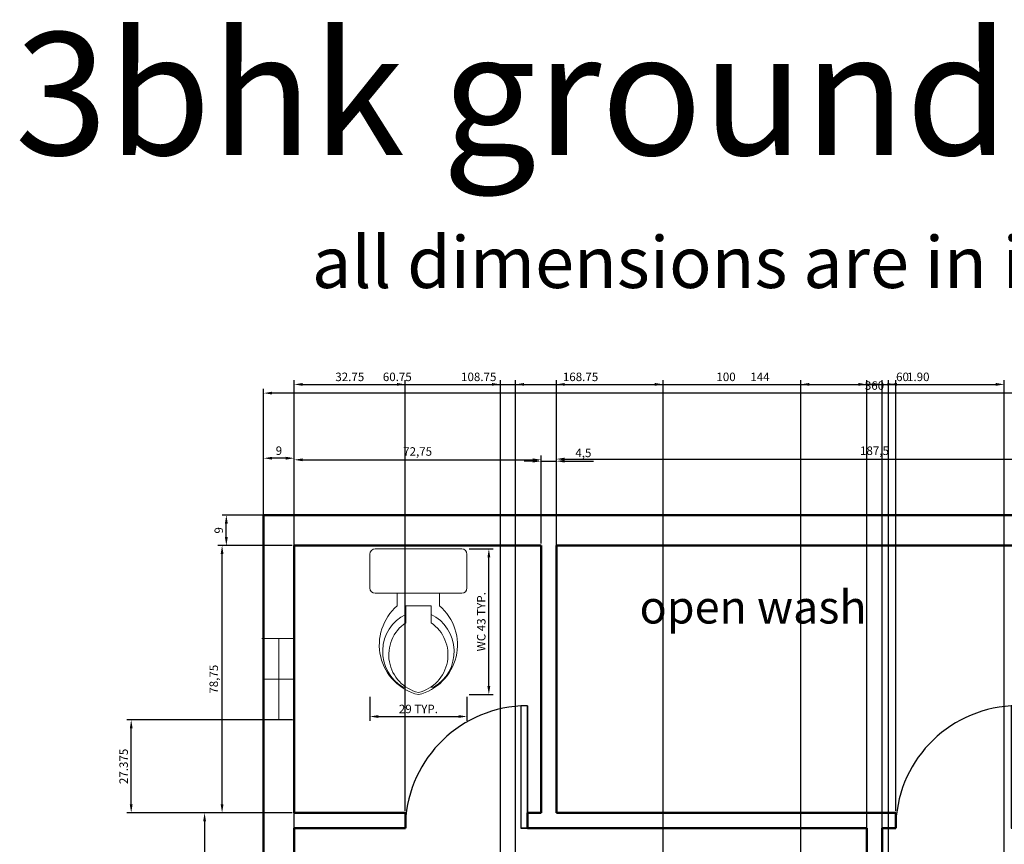
# Model space of a CAD drawing. Units: inches. Extents: x 907 to 2409, y 377 to 1163.
# Tile 6 of 9: x 907 to 1197, y 920 to 1163. Entities that reach past the tile are written whole.
import ezdxf

# ---------------------------------------------------------------- set-up
doc = ezdxf.new("R2010")
doc.units = ezdxf.units.IN
for name, color, linetype, lineweight in [('A-ANNO-DIMS', 2, 'Continuous', 18), ('A-ANNO-TEXT', 7, 'Continuous', 25), ('A-AREA-IDEN', 7, 'Continuous', 18), ('A-DOOR', 3, 'Continuous', 25), ('A-FLOR-FIXT', 9, 'Continuous', 18), ('A-GLAZ', 4, 'Continuous', 18), ('A-WALL', 7, 'Continuous', 50)]:
    doc.layers.add(name, color=color, linetype=linetype, lineweight=lineweight)
doc.styles.get("Standard").update_dxf_attribs({"font": 'arial.ttf'})
doc.dimstyles.new('ISO-25', dxfattribs={"dimtxt": 2.5, "dimasz": 2.5, "dimexe": 1.25, "dimexo": 0.625, "dimtad": 1, "dimtxsty": 'Standard', "dimcen": 2.5, "dimadec": 0, "dimazin": 0, "dimtfac": 1, "dimtmove": 0, "dimatfit": 3, "dimfxl": 1, "dimarcsym": 0})

# ---------------------------------------------------------------- blocks, each defined once
blk = doc.blocks.new('A$C02F3725D')
for p, q in [((0, 0.505), (0, 0.665)), ((0.025, 0.69), (0.435, 0.69)), ((0.46, 0.665), (0.46, 0.505)), ((0.435, 0.48), (0.025, 0.48)), ((0.13, 0.48), (0.13, 0.42)), ((0.33, 0.42), (0.33, 0.48)), ((0.17, 0.34), (0.17, 0.42)), ((0.17, 0.42), (0.29, 0.42)), ((0.29, 0.34), (0.29, 0.42)), ((0.1578, 0.035), (0.1724, 0.035)), ((0.2876, 0.035), (0.3022, 0.035))]:
    blk.add_line(p, q)
for centre, radius, start, end in [((0.025, 0.665), 0.025, 90, 180), ((0.435, 0.665), 0.025, 0, 90), ((0.025, 0.505), 0.025, 180, 270), ((0.435, 0.505), 0.025, 270, 0), ((0.2874, 0.2356), 0.2425, 130.4885, 256.2965), ((0.1726, 0.2356), 0.2425, 283.7035, 49.5115), ((0.2568, 0.2042), 0.196, 116.2742, 239.6668), ((0.2032, 0.2042), 0.196, 300.3332, 63.7258), ((0.2732, 0.1883), 0.1834, 124.2157, 256.394), ((0.1868, 0.1883), 0.1834, 283.606, 55.7843)]:
    blk.add_arc(centre, radius, start, end)
blk = doc.blocks.new('*D5')
at = {"layer": 'A-ANNO-DIMS', "color": 0, "lineweight": -2, "transparency": 16777216}
for p, q in [((978.61, 1008.5), (978.61, 1034.87)), ((985.11, 1033.62), (981.11, 1033.62)), ((987.61, 1008.5), (987.61, 1034.87))]:
    blk.add_line(p, q, dxfattribs=at)
at = {"layer": 'A-ANNO-DIMS', "color": 0, "transparency": 16777216}
for points in [[(981.11, 1034.04), (981.11, 1033.2), (978.61, 1033.62)], [(985.11, 1034.04), (985.11, 1033.2), (987.61, 1033.62)]]:
    blk.add_solid(points, dxfattribs=at)
at = {"layer": 'Defpoints', "color": 0, "transparency": 16777216}
for p in [(978.61, 1033.62), (978.61, 1007.87), (987.61, 1007.87)]:
    blk.add_point(p, dxfattribs=at)
at = {"layer": 'A-ANNO-DIMS', "color": 0, "transparency": 16777216, "insert": (983.11, 1035.52), "char_height": 2.5, "attachment_point": 5}
blk.add_mtext('9', dxfattribs=at)
blk = doc.blocks.new('*D6')
at = {"layer": 'A-ANNO-DIMS', "color": 0, "lineweight": -2, "transparency": 16777216}
for p, q in [((987.61, 1008.5), (987.61, 1034.4)), ((990.11, 1033.15), (1057.86, 1033.15)), ((1060.36, 1008.5), (1060.36, 1034.4))]:
    blk.add_line(p, q, dxfattribs=at)
at = {"layer": 'A-ANNO-DIMS', "color": 0, "transparency": 16777216}
for points in [[(990.11, 1033.57), (990.11, 1032.73), (987.61, 1033.15)], [(1057.86, 1033.57), (1057.86, 1032.73), (1060.36, 1033.15)]]:
    blk.add_solid(points, dxfattribs=at)
at = {"layer": 'Defpoints', "color": 0, "transparency": 16777216}
for p in [(1060.36, 1033.15), (987.61, 1007.87), (1060.36, 1007.87)]:
    blk.add_point(p, dxfattribs=at)
at = {"layer": 'A-ANNO-DIMS', "color": 0, "transparency": 16777216, "insert": (1023.99, 1035.28), "char_height": 2.5, "attachment_point": 5}
blk.add_mtext('72,75', dxfattribs=at)
blk = doc.blocks.new('*D7')
at = {"layer": 'A-ANNO-DIMS', "color": 0, "lineweight": -2, "transparency": 16777216}
for p, q in [((1060.36, 1008.5), (1060.36, 1034)), ((1064.86, 1008.5), (1064.86, 1034)), ((1057.86, 1032.75), (1055.36, 1032.75)), ((1060.36, 1032.75), (1064.86, 1032.75)), ((1067.36, 1032.75), (1075.78, 1032.75))]:
    blk.add_line(p, q, dxfattribs=at)
at = {"layer": 'A-ANNO-DIMS', "color": 0, "transparency": 16777216}
for points in [[(1057.86, 1033.16), (1057.86, 1032.33), (1060.36, 1032.75)], [(1067.36, 1033.16), (1067.36, 1032.33), (1064.86, 1032.75)]]:
    blk.add_solid(points, dxfattribs=at)
at = {"layer": 'Defpoints', "color": 0, "transparency": 16777216}
for p in [(1064.86, 1032.75), (1060.36, 1007.87), (1064.86, 1007.87)]:
    blk.add_point(p, dxfattribs=at)
at = {"layer": 'A-ANNO-DIMS', "color": 0, "transparency": 16777216, "insert": (1072.82, 1034.87), "char_height": 2.5, "attachment_point": 5}
blk.add_mtext('4,5', dxfattribs=at)
blk = doc.blocks.new('*D8')
at = {"layer": 'A-ANNO-DIMS', "color": 0, "lineweight": -2, "transparency": 16777216}
for p, q in [((1064.86, 1008.5), (1064.86, 1034.62)), ((1067.36, 1033.37), (1249.86, 1033.37)), ((1252.36, 1008.5), (1252.36, 1034.62))]:
    blk.add_line(p, q, dxfattribs=at)
at = {"layer": 'A-ANNO-DIMS', "color": 0, "transparency": 16777216}
for points in [[(1067.36, 1033.79), (1067.36, 1032.95), (1064.86, 1033.37)], [(1249.86, 1033.79), (1249.86, 1032.95), (1252.36, 1033.37)]]:
    blk.add_solid(points, dxfattribs=at)
at = {"layer": 'Defpoints', "color": 0, "transparency": 16777216}
for p in [(1252.36, 1033.37), (1064.86, 1007.87), (1252.36, 1007.87)]:
    blk.add_point(p, dxfattribs=at)
at = {"layer": 'A-ANNO-DIMS', "color": 0, "transparency": 16777216, "insert": (1158.61, 1035.5), "char_height": 2.5, "attachment_point": 5}
blk.add_mtext('187,5', dxfattribs=at)
blk = doc.blocks.new('*D12')
at = {"layer": 'A-ANNO-DIMS', "color": 0, "lineweight": -2, "transparency": 16777216}
for p, q in [((978.61, 1017.5), (978.61, 1054.05)), ((1338.61, 1017.5), (1338.61, 1054.05)), ((1336.11, 1052.8), (981.11, 1052.8))]:
    blk.add_line(p, q, dxfattribs=at)
at = {"layer": 'A-ANNO-DIMS', "color": 0, "transparency": 16777216}
for points in [[(981.11, 1053.22), (981.11, 1052.39), (978.61, 1052.8)], [(1336.11, 1053.22), (1336.11, 1052.39), (1338.61, 1052.8)]]:
    blk.add_solid(points, dxfattribs=at)
at = {"layer": 'Defpoints', "color": 0, "transparency": 16777216}
for p in [(978.61, 1052.8), (978.61, 1016.87), (1338.61, 1016.87)]:
    blk.add_point(p, dxfattribs=at)
at = {"layer": 'A-ANNO-DIMS', "color": 0, "transparency": 16777216, "insert": (1158.61, 1054.71), "char_height": 2.5, "attachment_point": 5}
blk.add_mtext('360', dxfattribs=at)
blk = doc.blocks.new('*D29')
at = {"layer": 'A-ANNO-DIMS', "color": 0, "lineweight": -2, "transparency": 16777216}
for p, q in [((986.99, 1016.87), (966.36, 1016.87)), ((967.61, 1010.37), (967.61, 1014.37)), ((986.99, 1007.87), (966.36, 1007.87))]:
    blk.add_line(p, q, dxfattribs=at)
at = {"layer": 'A-ANNO-DIMS', "color": 0, "transparency": 16777216}
for points in [[(967.19, 1014.37), (968.03, 1014.37), (967.61, 1016.87)], [(967.19, 1010.37), (968.03, 1010.37), (967.61, 1007.87)]]:
    blk.add_solid(points, dxfattribs=at)
at = {"layer": 'Defpoints', "color": 0, "transparency": 16777216}
for p in [(967.61, 1016.87), (987.61, 1016.87), (987.61, 1007.87)]:
    blk.add_point(p, dxfattribs=at)
at = {"layer": 'A-ANNO-DIMS', "color": 0, "transparency": 16777216, "insert": (965.71, 1012.37), "char_height": 2.5, "attachment_point": 5, "rotation": 90}
blk.add_mtext('9', dxfattribs=at)
blk = doc.blocks.new('*D30')
at = {"layer": 'A-ANNO-DIMS', "color": 0, "lineweight": -2, "transparency": 16777216}
for p, q in [((986.99, 1007.87), (965.11, 1007.87)), ((966.36, 931.62), (966.36, 1005.37)), ((986.99, 929.12), (965.11, 929.12))]:
    blk.add_line(p, q, dxfattribs=at)
at = {"layer": 'A-ANNO-DIMS', "color": 0, "transparency": 16777216}
for points in [[(965.94, 1005.37), (966.78, 1005.37), (966.36, 1007.87)], [(965.94, 931.62), (966.78, 931.62), (966.36, 929.12)]]:
    blk.add_solid(points, dxfattribs=at)
at = {"layer": 'Defpoints', "color": 0, "transparency": 16777216}
for p in [(966.36, 1007.87), (987.61, 1007.87), (987.61, 929.12)]:
    blk.add_point(p, dxfattribs=at)
at = {"layer": 'A-ANNO-DIMS', "color": 0, "transparency": 16777216, "insert": (964.23, 968.5), "char_height": 2.5, "attachment_point": 5, "rotation": 90}
blk.add_mtext('78,75', dxfattribs=at)
blk = doc.blocks.new('*D31')
at = {"layer": 'A-ANNO-DIMS', "color": 0, "lineweight": -2, "transparency": 16777216}
for p, q in [((986.99, 929.12), (959.95, 929.12)), ((961.2, 926.62), (961.2, 775.62)), ((986.99, 773.12), (959.95, 773.12))]:
    blk.add_line(p, q, dxfattribs=at)
at = {"layer": 'A-ANNO-DIMS', "color": 0, "transparency": 16777216}
for points in [[(960.78, 926.62), (961.62, 926.62), (961.2, 929.12)], [(960.78, 775.62), (961.62, 775.62), (961.2, 773.12)]]:
    blk.add_solid(points, dxfattribs=at)
at = {"layer": 'Defpoints', "color": 0, "transparency": 16777216}
for p in [(987.61, 929.12), (961.2, 773.12), (987.61, 773.12)]:
    blk.add_point(p, dxfattribs=at)
at = {"layer": 'A-ANNO-DIMS', "color": 0, "transparency": 16777216, "insert": (959.3, 851.12), "char_height": 2.5, "attachment_point": 5, "rotation": 90}
blk.add_mtext('156', dxfattribs=at)
blk = doc.blocks.new('DOOR-36IN')
for p, q in [((36, 36), (36, 0)), ((36, 0), (34, 0)), ((36, 0), (34, 0))]:
    blk.add_line(p, q)
blk.add_lwpolyline([(36, 36), (34, 36), (34, 0), (36, 0)], close=True)
blk.add_arc((36.06, 0), 36.06, 93.2732, 180)
blk = doc.blocks.new('WIN-24IN')
for p, q in [((0.53, 23.99), (0, 23.99)), ((9.53, 24), (0.53, 24)), ((5.03, 0), (5.03, 24)), ((9.53, 12), (0.53, 12)), ((9.53, 0), (0.53, 0))]:
    blk.add_line(p, q)
blk = doc.blocks.new('*D49')
at = {"layer": 'A-ANNO-DIMS', "color": 0, "lineweight": -2, "transparency": 16777216}
for p, q in [((1039.15, 1006.91), (1046.22, 1006.91)), ((1044.97, 966.46), (1044.97, 1004.41)), ((1039.15, 963.96), (1046.22, 963.96))]:
    blk.add_line(p, q, dxfattribs=at)
at = {"layer": 'A-ANNO-DIMS', "color": 0, "transparency": 16777216}
for points in [[(1044.55, 1004.41), (1045.39, 1004.41), (1044.97, 1006.91)], [(1044.55, 966.46), (1045.39, 966.46), (1044.97, 963.96)]]:
    blk.add_solid(points, dxfattribs=at)
at = {"layer": 'Defpoints', "color": 0, "transparency": 16777216}
for p in [(1038.53, 1006.91), (1044.97, 1006.91), (1038.53, 963.96)]:
    blk.add_point(p, dxfattribs=at)
at = {"layer": 'A-ANNO-DIMS', "color": 0, "transparency": 16777216, "insert": (1043.05, 985.43), "char_height": 2.5, "attachment_point": 5, "rotation": 90}
blk.add_mtext('WC 43 TYP.', dxfattribs=at)
blk = doc.blocks.new('*D50')
at = {"layer": 'A-ANNO-DIMS', "color": 0, "lineweight": -2, "transparency": 16777216}
for p, q in [((1009.89, 963.33), (1009.89, 956.26)), ((1038.53, 963.33), (1038.53, 956.26)), ((1012.39, 957.51), (1036.03, 957.51))]:
    blk.add_line(p, q, dxfattribs=at)
at = {"layer": 'A-ANNO-DIMS', "color": 0, "transparency": 16777216}
for points in [[(1012.39, 957.93), (1012.39, 957.1), (1009.89, 957.51)], [(1036.03, 957.93), (1036.03, 957.1), (1038.53, 957.51)]]:
    blk.add_solid(points, dxfattribs=at)
at = {"layer": 'Defpoints', "color": 0, "transparency": 16777216}
for p in [(1009.89, 963.96), (1038.53, 963.96), (1038.53, 957.51)]:
    blk.add_point(p, dxfattribs=at)
at = {"layer": 'A-ANNO-DIMS', "color": 0, "transparency": 16777216, "insert": (1024.21, 959.42), "char_height": 2.5, "attachment_point": 5}
blk.add_mtext('29 TYP.', dxfattribs=at)
blk = doc.blocks.new('*D59')
at = {"layer": 'A-ANNO-DIMS', "color": 0, "lineweight": -2, "transparency": 16777216}
for p, q in [((987.61, 773.75), (987.61, 1056.62)), ((1156.36, 773.75), (1156.36, 1056.62)), ((990.11, 1055.37), (1153.86, 1055.37))]:
    blk.add_line(p, q, dxfattribs=at)
at = {"layer": 'A-ANNO-DIMS', "color": 0, "transparency": 16777216}
for points in [[(990.11, 1055.79), (990.11, 1054.95), (987.61, 1055.37)], [(1153.86, 1055.79), (1153.86, 1054.95), (1156.36, 1055.37)]]:
    blk.add_solid(points, dxfattribs=at)
at = {"layer": 'Defpoints', "color": 0, "transparency": 16777216}
for p in [(1156.36, 1055.37), (987.61, 773.12), (1156.36, 773.12)]:
    blk.add_point(p, dxfattribs=at)
at = {"layer": 'A-ANNO-DIMS', "color": 0, "transparency": 16777216, "insert": (1071.99, 1057.27), "char_height": 2.5, "attachment_point": 5}
blk.add_mtext('168.75', dxfattribs=at)
blk = doc.blocks.new('*D60')
at = {"layer": 'A-ANNO-DIMS', "color": 0, "lineweight": -2, "transparency": 16777216}
for p, q in [((987.61, 689.75), (987.61, 1056.62)), ((1048.36, 689.75), (1048.36, 1056.62)), ((990.11, 1055.37), (1045.86, 1055.37))]:
    blk.add_line(p, q, dxfattribs=at)
at = {"layer": 'A-ANNO-DIMS', "color": 0, "transparency": 16777216}
for points in [[(990.11, 1055.79), (990.11, 1054.95), (987.61, 1055.37)], [(1045.86, 1055.79), (1045.86, 1054.95), (1048.36, 1055.37)]]:
    blk.add_solid(points, dxfattribs=at)
at = {"layer": 'Defpoints', "color": 0, "transparency": 16777216}
for p in [(1048.36, 1055.37), (987.61, 689.12), (1048.36, 689.12)]:
    blk.add_point(p, dxfattribs=at)
at = {"layer": 'A-ANNO-DIMS', "color": 0, "transparency": 16777216, "insert": (1017.99, 1057.27), "char_height": 2.5, "attachment_point": 5}
blk.add_mtext('60.75', dxfattribs=at)
blk = doc.blocks.new('*D61')
at = {"layer": 'A-ANNO-DIMS', "color": 0, "lineweight": -2, "transparency": 16777216}
for p, q in [((1052.86, 729.25), (1052.86, 1056.62)), ((1196.86, 727.25), (1196.86, 1056.62)), ((1055.36, 1055.37), (1194.36, 1055.37))]:
    blk.add_line(p, q, dxfattribs=at)
at = {"layer": 'A-ANNO-DIMS', "color": 0, "transparency": 16777216}
for points in [[(1055.36, 1055.79), (1055.36, 1054.95), (1052.86, 1055.37)], [(1194.36, 1055.79), (1194.36, 1054.95), (1196.86, 1055.37)]]:
    blk.add_solid(points, dxfattribs=at)
at = {"layer": 'Defpoints', "color": 0, "transparency": 16777216}
for p in [(1196.86, 1055.37), (1052.86, 728.62), (1196.86, 726.62)]:
    blk.add_point(p, dxfattribs=at)
at = {"layer": 'A-ANNO-DIMS', "color": 0, "transparency": 16777216, "insert": (1124.86, 1057.25), "char_height": 2.5, "attachment_point": 5}
blk.add_mtext('144', dxfattribs=at)
blk = doc.blocks.new('*D62')
at = {"layer": 'A-ANNO-DIMS', "color": 0, "lineweight": -2, "transparency": 16777216}
for p, q in [((987.61, 426.5), (987.61, 1056.62)), ((1096.36, 426.5), (1096.36, 1056.62)), ((990.11, 1055.37), (1093.86, 1055.37))]:
    blk.add_line(p, q, dxfattribs=at)
at = {"layer": 'A-ANNO-DIMS', "color": 0, "transparency": 16777216}
for points in [[(990.11, 1055.79), (990.11, 1054.95), (987.61, 1055.37)], [(1093.86, 1055.79), (1093.86, 1054.95), (1096.36, 1055.37)]]:
    blk.add_solid(points, dxfattribs=at)
at = {"layer": 'Defpoints', "color": 0, "transparency": 16777216}
for p in [(1096.36, 1055.37), (987.61, 425.87), (1096.36, 425.87)]:
    blk.add_point(p, dxfattribs=at)
at = {"layer": 'A-ANNO-DIMS', "color": 0, "transparency": 16777216, "insert": (1041.99, 1057.27), "char_height": 2.5, "attachment_point": 5}
blk.add_mtext('108.75', dxfattribs=at)
blk = doc.blocks.new('*D66')
at = {"layer": 'A-ANNO-DIMS', "color": 0, "lineweight": -2, "transparency": 16777216}
for p, q in [((1064.86, 929.75), (1064.86, 1056.62)), ((1164.86, 929.75), (1164.86, 1056.62)), ((1067.36, 1055.37), (1162.36, 1055.37))]:
    blk.add_line(p, q, dxfattribs=at)
at = {"layer": 'A-ANNO-DIMS', "color": 0, "transparency": 16777216}
for points in [[(1067.36, 1055.79), (1067.36, 1054.95), (1064.86, 1055.37)], [(1162.36, 1055.79), (1162.36, 1054.95), (1164.86, 1055.37)]]:
    blk.add_solid(points, dxfattribs=at)
at = {"layer": 'Defpoints', "color": 0, "transparency": 16777216}
for p in [(1164.86, 1055.37), (1064.86, 929.12), (1164.86, 929.12)]:
    blk.add_point(p, dxfattribs=at)
at = {"layer": 'A-ANNO-DIMS', "color": 0, "transparency": 16777216, "insert": (1114.86, 1057.27), "char_height": 2.5, "attachment_point": 5}
blk.add_mtext('100', dxfattribs=at)
blk = doc.blocks.new('*D67')
at = {"layer": 'A-ANNO-DIMS', "color": 0, "lineweight": -2, "transparency": 16777216}
for p, q in [((987.61, 929.75), (987.61, 1056.62)), ((1020.36, 929.75), (1020.36, 1056.62)), ((990.11, 1055.37), (1017.86, 1055.37))]:
    blk.add_line(p, q, dxfattribs=at)
at = {"layer": 'A-ANNO-DIMS', "color": 0, "transparency": 16777216}
for points in [[(990.11, 1055.79), (990.11, 1054.95), (987.61, 1055.37)], [(1017.86, 1055.79), (1017.86, 1054.95), (1020.36, 1055.37)]]:
    blk.add_solid(points, dxfattribs=at)
at = {"layer": 'Defpoints', "color": 0, "transparency": 16777216}
for p in [(1020.36, 1055.37), (987.61, 929.12), (1020.36, 929.12)]:
    blk.add_point(p, dxfattribs=at)
at = {"layer": 'A-ANNO-DIMS', "color": 0, "transparency": 16777216, "insert": (1003.99, 1057.27), "char_height": 2.5, "attachment_point": 5}
blk.add_mtext('32.75', dxfattribs=at)
blk = doc.blocks.new('*D70')
at = {"layer": 'A-ANNO-DIMS', "color": 0, "lineweight": -2, "transparency": 16777216}
for p, q in [((986.99, 956.5), (938.33, 956.5)), ((939.58, 931.62), (939.58, 954)), ((986.99, 929.12), (938.33, 929.12))]:
    blk.add_line(p, q, dxfattribs=at)
at = {"layer": 'A-ANNO-DIMS', "color": 0, "transparency": 16777216}
for points in [[(939.17, 954), (940, 954), (939.58, 956.5)], [(939.17, 931.62), (940, 931.62), (939.58, 929.12)]]:
    blk.add_solid(points, dxfattribs=at)
at = {"layer": 'Defpoints', "color": 0, "transparency": 16777216}
for p in [(939.58, 956.5), (987.61, 956.5), (987.61, 929.12)]:
    blk.add_point(p, dxfattribs=at)
at = {"layer": 'A-ANNO-DIMS', "color": 0, "transparency": 16777216, "insert": (937.68, 942.81), "char_height": 2.5, "attachment_point": 5, "rotation": 90}
blk.add_mtext('27.375', dxfattribs=at)
blk = doc.blocks.new('*D75')
at = {"layer": 'A-ANNO-DIMS', "color": 0, "lineweight": -2, "transparency": 16777216}
for p, q in [((1136.86, 613.25), (1136.86, 1056.62)), ((1196.86, 613.25), (1196.86, 1056.62)), ((1139.36, 1055.37), (1194.36, 1055.37))]:
    blk.add_line(p, q, dxfattribs=at)
at = {"layer": 'A-ANNO-DIMS', "color": 0, "transparency": 16777216}
for points in [[(1139.36, 1055.79), (1139.36, 1054.95), (1136.86, 1055.37)], [(1194.36, 1055.79), (1194.36, 1054.95), (1196.86, 1055.37)]]:
    blk.add_solid(points, dxfattribs=at)
at = {"layer": 'Defpoints', "color": 0, "transparency": 16777216}
for p in [(1196.86, 1055.37), (1136.86, 612.62), (1196.86, 612.62)]:
    blk.add_point(p, dxfattribs=at)
at = {"layer": 'A-ANNO-DIMS', "color": 0, "transparency": 16777216, "insert": (1166.86, 1057.27), "char_height": 2.5, "attachment_point": 5}
blk.add_mtext('60', dxfattribs=at)
blk = doc.blocks.new('*D85')
at = {"layer": 'A-ANNO-DIMS', "color": 0, "lineweight": -2, "transparency": 16777216}
for p, q in [((1160.86, 773.75), (1160.86, 1056.62)), ((1162.76, 773.75), (1162.76, 1056.62)), ((1158.36, 1055.37), (1155.86, 1055.37)), ((1160.86, 1055.37), (1162.76, 1055.37)), ((1165.26, 1055.37), (1175.26, 1055.37))]:
    blk.add_line(p, q, dxfattribs=at)
at = {"layer": 'A-ANNO-DIMS', "color": 0, "transparency": 16777216}
for points in [[(1158.36, 1055.79), (1158.36, 1054.95), (1160.86, 1055.37)], [(1165.26, 1055.79), (1165.26, 1054.95), (1162.76, 1055.37)]]:
    blk.add_solid(points, dxfattribs=at)
at = {"layer": 'Defpoints', "color": 0, "transparency": 16777216}
for p in [(1162.76, 1055.37), (1160.86, 773.12), (1162.76, 773.12)]:
    blk.add_point(p, dxfattribs=at)
at = {"layer": 'A-ANNO-DIMS', "color": 0, "transparency": 16777216, "insert": (1171.51, 1057.27), "char_height": 2.5, "attachment_point": 5}
blk.add_mtext('1.90', dxfattribs=at)

msp = doc.modelspace()

# ---------------------------------------------------------------- linework, layer by layer
at = {"layer": 'A-WALL'}
for p, q in [((978.6122, 1016.8705), (1338.6122, 1016.8705)), ((978.6122, 1016.8705), (978.6122, 926.8705)), ((978.6122, 1016.8705), (978.6122, 416.8705)), ((978.6122, 1016.8705), (1338.6122, 1016.8705)), ((987.6122, 1007.8705), (1060.3622, 1007.8705)), ((987.6122, 1007.8705), (987.6122, 929.1205)), ((1060.3622, 1007.8705), (1060.3622, 929.1205)), ((1064.8622, 1007.8705), (1064.8622, 929.1205)), ((1064.8622, 1007.8705), (1252.3622, 1007.8705)), ((1064.8622, 1007.8705), (1252.3622, 1007.8705)), ((987.6122, 929.1205), (1020.3622, 929.1205)), ((1020.3622, 929.1205), (1020.3622, 924.6205)), ((1056.3622, 929.1205), (1056.3622, 924.6205)), ((1056.3622, 929.1205), (1060.3622, 929.1205)), ((1064.8622, 929.1205), (1164.8622, 929.1205)), ((1164.8622, 924.6205), (1164.8622, 929.1205)), ((978.6122, 926.8705), (978.6122, 770.8705)), ((987.6122, 924.6205), (1020.3622, 924.6205)), ((987.6122, 924.6205), (987.6122, 773.1205)), ((1056.3622, 924.6205), (1156.3622, 924.6205)), ((1156.3622, 924.6205), (1156.3622, 773.1205)), ((1160.8622, 924.6205), (1160.8622, 773.1205)), ((1160.8622, 924.6205), (1164.8622, 924.6205))]:
    msp.add_line(p, q, dxfattribs=at)
msp.add_lwpolyline([(1216.3622, 416.8705), (1338.6122, 416.8705), (1338.6122, 1016.8705), (978.6122, 1016.8705), (978.6122, 416.8705), (1100.8622, 416.8705)], dxfattribs=at)

# ---------------------------------------------------------------- block references
at = {"layer": 'A-DOOR'}
for p in [(1020.3622, 924.6205), (1164.8622, 924.6205)]:
    msp.add_blockref('DOOR-36IN', p, dxfattribs=at)
at = {"layer": 'A-FLOR-FIXT', "xscale": 62.24890487658392, "yscale": 62.24890487658392, "zscale": 62.24890487658392}
msp.add_blockref('A$C02F3725D', (1009.8918, 963.9577), dxfattribs=at)
at = {"layer": 'A-GLAZ'}
msp.add_blockref('WIN-24IN', (978.083, 956.496), dxfattribs=at)

# ---------------------------------------------------------------- texts
at = {"layer": 'A-ANNO-TEXT', "attachment_point": 1}
for s, width, gutter_width, insert, char_height in [('3bhk ground floor plan', 591.346782, 180.477, (905.2958, 1159.0854), 36.095399), ('all dimensions are in inches', 399.634663, 75.8973, (992.819, 1098.9518), 15.179467)]:
    msp.add_mtext_dynamic_manual_height_columns(s, width=width, gutter_width=gutter_width, heights=[0], dxfattribs=dict(at, insert=insert, char_height=char_height))
at = {"layer": 'A-AREA-IDEN', "insert": (1089.3805, 994.6243), "char_height": 9.70457, "attachment_point": 1}
msp.add_mtext('open wash', dxfattribs=at)

# ---------------------------------------------------------------- dimensions: what is measured, and where the dimension line sits
at = {"layer": 'A-ANNO-DIMS'}
for base, p1, p2, override, picture, middle in [((978.6122, 1052.8035), (1338.6122, 1016.8705), (978.6122, 1016.8705), {"dimclrd": 0, "dimclre": 0, "dimclrt": 0}, '*D12', (1158.6122, 1054.7058)), ((1020.3622, 1055.3705), (987.6122, 929.1205), (1020.3622, 929.1205), {"dimdec": 2, "dimlfac": 1, "dimrnd": 0, "dimzin": 0, "dimdsep": 46, "dimlunit": 2}, '*D67', (1003.9872, 1057.2728)), ((1156.3622, 1055.3705), (987.6122, 773.1205), (1156.3622, 773.1205), {"dimdec": 2, "dimlfac": 1, "dimrnd": 0, "dimzin": 0, "dimdsep": 46, "dimlunit": 2}, '*D59', (1071.9872, 1057.272)), ((1048.3622, 1055.3705), (987.6122, 689.1205), (1048.3622, 689.1205), {"dimdec": 2, "dimlfac": 1, "dimrnd": 0, "dimzin": 0, "dimdsep": 46, "dimlunit": 2}, '*D60', (1017.9872, 1057.272)), ((1096.3622, 1055.3705), (987.6122, 425.8705), (1096.3622, 425.8705), {"dimdec": 2, "dimlfac": 1, "dimrnd": 0, "dimzin": 0, "dimdsep": 46, "dimlunit": 2}, '*D62', (1041.9872, 1057.272)), ((1196.8622, 1055.3705), (1052.8622, 728.6205), (1196.8622, 726.6205), {"dimdec": 0, "dimlfac": 1, "dimrnd": 0, "dimzin": 0, "dimdsep": 46, "dimlunit": 2}, '*D61', (1124.8622, 1057.2507)), ((1164.8622, 1055.3705), (1064.8622, 929.1205), (1164.8622, 929.1205), {"dimdec": 0, "dimlfac": 1, "dimrnd": 0, "dimzin": 0, "dimdsep": 46, "dimlunit": 2}, '*D66', (1114.8622, 1057.272)), ((1196.8622, 1055.3705), (1136.8622, 612.6205), (1196.8622, 612.6205), {"dimdec": 0, "dimlfac": 1, "dimrnd": 0, "dimzin": 0, "dimdsep": 46, "dimlunit": 2}, '*D75', (1166.8622, 1057.272)), ((1162.7586, 1055.3705), (1160.8622, 773.1205), (1162.7586, 773.1205), {"dimdec": 2, "dimlfac": 1, "dimrnd": 0, "dimzin": 0, "dimdsep": 46, "dimlunit": 2}, '*D85', (1171.5086, 1057.272)), ((978.6122, 1033.6191), (987.6122, 1007.8705), (978.6122, 1007.8705), {"dimclrd": 0, "dimclre": 0, "dimclrt": 0}, '*D5', (983.1122, 1035.5206)), ((1060.3622, 1033.1513), (987.6122, 1007.8705), (1060.3622, 1007.8705), {"dimclrd": 0, "dimclre": 0, "dimclrt": 0}, '*D6', (1023.9872, 1035.2787)), ((1064.8622, 1032.7463), (1060.3622, 1007.8705), (1064.8622, 1007.8705), {"dimclrd": 0, "dimclre": 0, "dimclrt": 0}, '*D7', (1072.8227, 1034.8686)), ((1252.3622, 1033.3713), (1064.8622, 1007.8705), (1252.3622, 1007.8705), {"dimclrd": 0, "dimclre": 0, "dimclrt": 0}, '*D8', (1158.6122, 1035.4987))]:
    dim = msp.add_linear_dim(base=base, p1=p1, p2=p2, dimstyle='ISO-25', override=override, dxfattribs=at)
    dim.commit()
    dim.dimension.update_dxf_attribs({"geometry": picture, "text_midpoint": middle})
for base, p1, p2, override, picture, middle in [((967.6091, 1016.8705), (987.6122, 1007.8705), (987.6122, 1016.8705), {"dimclrd": 0, "dimclre": 0, "dimclrt": 0}, '*D29', (965.7077, 1012.3705)), ((966.3591, 1007.8705), (987.6122, 929.1205), (987.6122, 1007.8705), {"dimclrd": 0, "dimclre": 0, "dimclrt": 0}, '*D30', (964.2318, 968.4955)), ((939.5829, 956.4955), (987.6122, 929.1205), (987.6122, 956.4955), {"dimdec": 3, "dimlfac": 1, "dimrnd": 0, "dimzin": 0, "dimdsep": 46, "dimlunit": 2}, '*D70', (937.6807, 942.808)), ((961.1988, 773.1205), (987.6122, 929.1205), (987.6122, 773.1205), {"dimclrd": 0, "dimclre": 0, "dimclrt": 0}, '*D31', (959.2973, 851.1205))]:
    dim = msp.add_linear_dim(base=base, p1=p1, p2=p2, angle=90, dimstyle='ISO-25', override=override, dxfattribs=at)
    dim.commit()
    dim.dimension.update_dxf_attribs({"geometry": picture, "text_midpoint": middle})
dim = msp.add_linear_dim(base=(1044.969, 1006.9095), p1=(1038.5263, 963.9577), p2=(1038.5263, 1006.9095), angle=90, text='WC <> TYP.', dimstyle='ISO-25', override={"dimdec": 0, "dimlfac": 1, "dimrnd": 0, "dimzin": 0, "dimdsep": 46, "dimlunit": 2}, dxfattribs=at)
dim.commit()
dim.dimension.update_dxf_attribs({"geometry": '*D49', "text_midpoint": (1043.0505, 985.4336)})
dim = msp.add_linear_dim(base=(1038.5263, 957.515), p1=(1009.8918, 963.9577), p2=(1038.5263, 963.9577), text='<> TYP.', dimstyle='ISO-25', override={"dimdec": 0, "dimlfac": 1, "dimrnd": 0, "dimzin": 0, "dimdsep": 46, "dimlunit": 2}, dxfattribs=at)
dim.commit()
dim.dimension.update_dxf_attribs({"geometry": '*D50', "text_midpoint": (1024.209, 959.4164)})

doc.saveas('drawing.dxf')
